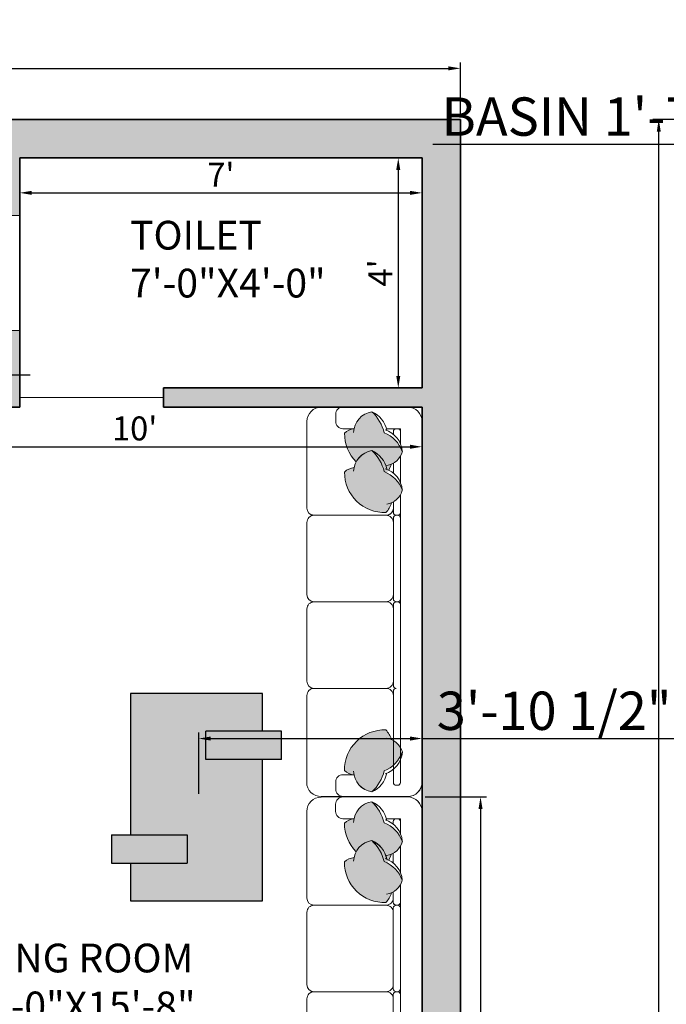
# Model space of a CAD drawing. Units: inches. Extents: x 3259 to 4981, y 1402 to 2026.
# Tile 4 of 11: x 3509 to 3644, y 1722 to 1928. Entities that reach past the tile are written whole.
import ezdxf

# ---------------------------------------------------------------- set-up
doc = ezdxf.new("R2010")
doc.units = ezdxf.units.IN
for name, color, linetype, lineweight in [('A-ANNO-DIMS', 2, 'Continuous', 13), ('A-AREA-IDEN', 7, 'Continuous', 18), ('A-DOOR', 3, 'Continuous', 18), ('A-FURN', 8, 'Continuous', 13), ('A-GLAZ', 4, 'Continuous', 18), ('A-WALL', 7, 'Continuous', 35), ('A-WALL-PATT', 252, 'Continuous', 13), ('parede', 7, 'Continuous', 30)]:
    doc.layers.add(name, color=color, linetype=linetype, lineweight=lineweight)
doc.styles.get("Standard").update_dxf_attribs({"font": 'arial.ttf'})
doc.dimstyles.new('ISO-25', dxfattribs={"dimtxt": 8, "dimasz": 2.5, "dimexe": 1.25, "dimexo": 0.625, "dimtad": 1, "dimdec": 1, "dimlunit": 3, "dimtxsty": 'Standard', "dimcen": 2.5, "dimclrd": 4, "dimclre": 4, "dimclrt": 1, "dimadec": 0, "dimazin": 0, "dimtfac": 1, "dimtdec": 1, "dimtmove": 0, "dimatfit": 3, "dimfxl": 1, "dimarcsym": 0})

# ---------------------------------------------------------------- blocks, each defined once
blk = doc.blocks.new('SOFA 1')
at = {"transparency": 33554687}
h = blk.add_hatch(color=256, dxfattribs=at)
h.dxf.hatch_style = 1
h.paths.add_polyline_path([(3769.65, 1307.6, 0.084911), (3767.15, 1309.12, 0.046133), (3766.46, 1311.13), (3759.18, 1311.13, 0.039409), (3758.92, 1310.24, 0.165523), (3756.31, 1309.02, 0.42585), (3767.59, 1297.95, 0.121928), (3769.15, 1300.58, 0.027403), (3769.65, 1300.83)])
h.paths.add_polyline_path([(3765.34, 1313.08), (3760.4, 1313.08, 0.097704), (3759.18, 1311.13), (3766.46, 1311.13, 0.04873)])
h.paths.add_polyline_path([(3763.76, 1314.88, 0.16488), (3760.4, 1313.08), (3765.34, 1313.08, 0.051917)])
h.paths.add_polyline_path([(3771.6, 1305.17, 0.090388), (3769.65, 1307.6), (3769.65, 1300.83, 0.136035), (3771.6, 1302.77)])
h = blk.add_hatch(color=256, dxfattribs=at)
h.dxf.hatch_style = 1
h.paths.add_polyline_path([(3723.52, 1308.63, 0.147724), (3717.76, 1305.24, 0.310469), (3722.42, 1300.4), (3722.42, 1300.25, 0.156703), (3723.62, 1297.8, 0.425821), (3734.69, 1309.08, 0.121928), (3732.05, 1310.63, 0.233216), (3728.6, 1313.59, 0.213835)])
h = blk.add_hatch(color=256, dxfattribs=at)
h.dxf.hatch_style = 1
h.paths.add_polyline_path([(3769.16, 1235.96, 0.122267), (3767.6, 1238.61, 0.425972), (3756.32, 1227.54, 0.165563), (3758.93, 1226.32, 0.309481), (3763.76, 1221.69, 0.002677), (3763.83, 1221.72, 0.146094), (3767.16, 1227.43, 0.212433), (3772.1, 1232.48, 0.235342)])
h = blk.add_hatch(color=256, dxfattribs=at)
h.dxf.hatch_style = 1
h.paths.add_polyline_path([(3769.16, 1225.36, 0.122267), (3767.6, 1228.01, 0.425972), (3756.32, 1216.94, 0.165563), (3758.93, 1215.72, 0.309481), (3763.76, 1211.09, 0.002677), (3763.83, 1211.12, 0.146094), (3767.16, 1216.83, 0.212433), (3772.1, 1221.88, 0.235342)])
for p, q in [((3720.45, 1316.13), (3773.58, 1316.13)), ((3777.51, 1312.19), (3777.51, 1213.72))]:
    blk.add_line(p, q, dxfattribs=at)
for points in [[(3763.76, 1314.88, -0.147724), (3767.15, 1309.12, -0.213355), (3772.1, 1304.05, 0.213355), (3767.15, 1309.12, 0.147724), (3763.76, 1314.88, -0.249545), (3767.86, 1309.77, 0.249545), (3763.77, 1314.89, 0.356779), (3758.8, 1309.23, -0.356779), (3763.76, 1314.88)], [(3717.76, 1305.24, -0.147724), (3723.52, 1308.63, -0.213355), (3728.59, 1313.59, 0.213355), (3723.52, 1308.63, 0.147724), (3717.76, 1305.24, -0.249545), (3722.86, 1309.34, 0.249545), (3717.75, 1305.25, 0.356779), (3723.4, 1300.28, -0.356779), (3717.76, 1305.24)], [(3728.58, 1313.6, -0.306333), (3732.42, 1309.31, 0.306333), (3728.58, 1313.6, 0.306674), (3722.72, 1308.89, -0.306674), (3728.58, 1313.6)], [(3734.69, 1309.08, -0.425972), (3723.62, 1297.8, -0.165552), (3722.4, 1300.4, 0.165552), (3723.62, 1297.79, 0.425972), (3734.69, 1309.07, 0.121514), (3732.07, 1310.63, -0.121514), (3734.69, 1309.08)], [(3767.6, 1297.95, -0.425972), (3756.31, 1309.01, -0.165552), (3758.92, 1310.24, 0.165552), (3756.31, 1309.02, 0.425972), (3767.59, 1297.95, 0.121514), (3769.14, 1300.57, -0.121514), (3767.6, 1297.95)], [(3772.11, 1304.06, -0.306333), (3767.83, 1300.22, 0.306333), (3772.11, 1304.06, 0.306674), (3767.4, 1309.91, -0.306674), (3772.11, 1304.06)], [(3770.44, 1286.63, -0.414214), (3769.66, 1287.4, 0.414214), (3770.44, 1286.63, 0.414214), (3769.66, 1285.83, -0.414214), (3770.44, 1286.63)], [(3748.01, 1262.99, -0.414214), (3746.05, 1264.95, 0.414214), (3748.01, 1262.97, 0.414213), (3746.05, 1261.01, -0.414213), (3748.01, 1262.99)], [(3770.44, 1262.99, -0.414214), (3769.66, 1263.77, 0.414214), (3770.44, 1262.99, 0.414214), (3769.66, 1262.19, -0.414214), (3770.44, 1262.99)], [(3770.83, 1262.97, -0.414214), (3771.61, 1262.19, 0.414214), (3770.83, 1262.99, 0.414214), (3771.61, 1263.77, -0.414214), (3770.83, 1262.97)], [(3748.01, 1239.35, -0.414214), (3746.05, 1241.31, 0.414214), (3748.01, 1239.33, 0.414213), (3746.05, 1237.37, -0.414213), (3748.01, 1239.35)], [(3767.7, 1239.33, -0.414214), (3769.66, 1237.37, 0.414214), (3767.7, 1239.35, 0.414214), (3769.66, 1241.31, -0.414214), (3767.7, 1239.33)], [(3770.44, 1239.35, -0.414214), (3769.66, 1240.13, 0.414214), (3770.44, 1239.33, 0.414214), (3769.66, 1238.55, -0.414214), (3770.44, 1239.35)], [(3770.83, 1239.33, -0.414214), (3771.61, 1238.55, 0.414214), (3770.83, 1239.35, 0.414214), (3771.61, 1240.13, -0.414214), (3770.83, 1239.33)], [(3756.32, 1227.54, -0.425972), (3767.6, 1238.61, -0.121514), (3769.16, 1235.98, 0.121514), (3767.6, 1238.61, 0.425972), (3756.32, 1227.54, 0.165552), (3758.93, 1226.32, -0.165552), (3756.32, 1227.54)], [(3772.1, 1232.5, -0.306674), (3767.41, 1226.64, 0.306674), (3772.1, 1232.5, 0.306333), (3767.84, 1236.34, -0.306333), (3772.1, 1232.5)], [(3763.78, 1221.67, 0.249545), (3767.87, 1226.78, -0.249545), (3763.76, 1221.69, -0.356779), (3758.81, 1227.32, 0.356779), (3763.77, 1221.68, 0.147724), (3767.16, 1227.43, 0.213355), (3772.11, 1232.51, -0.213355), (3767.16, 1227.43, -0.147724), (3763.78, 1221.67)], [(3756.32, 1216.94, -0.200233), (3759.49, 1224.76, 0.200233), (3756.32, 1216.94, 0.165552), (3758.93, 1215.72, -0.165552), (3756.32, 1216.94)], [(3772.1, 1221.9, -0.306674), (3767.41, 1216.04, 0.306674), (3772.1, 1221.9, -0.213355), (3767.16, 1216.83, -0.147724), (3763.77, 1211.08, 0.147724), (3767.15, 1216.83, 0.213355), (3772.1, 1221.9)], [(3763.76, 1211.09, -0.356779), (3758.81, 1216.72, 0.356779), (3763.76, 1211.09, 0.249545), (3767.87, 1216.18, -0.249545), (3763.76, 1211.09)]]:
    blk.add_lwpolyline(points, format="xyb", dxfattribs=at)
for points in [[(3716.51, 1312.2), (3716.51, 1291.44)], [(3722.42, 1313.08), (3722.42, 1309.23), (3722.42, 1313.08), (3726.57, 1313.08)], [(3729.85, 1313.08), (3745.25, 1313.08)], [(3746.01, 1312.3), (3746.01, 1288.55)], [(3768.11, 1313.08), (3746.78, 1313.08)], [(3771.6, 1313.08), (3767.75, 1313.08), (3771.6, 1313.08), (3771.6, 1308.93)], [(3769.66, 1287.39), (3769.65, 1312.3)], [(3771.6, 1313.08), (3771.61, 1233.74)], [(3723.21, 1311.13), (3723.93, 1311.13)], [(3731.82, 1311.13), (3745.25, 1311.13)], [(3746.01, 1310.97), (3746.01, 1311.36)], [(3768.87, 1311.13), (3746.78, 1311.13)], [(3769.65, 1309.43), (3769.65, 1308.71)], [(3746.01, 1288.54), (3746.01, 1308.23)], [(3722.42, 1300.39), (3722.42, 1297.33)], [(3720.45, 1295.38), (3718.48, 1295.38)], [(3720.45, 1287.5), (3744.09, 1287.5)], [(3747.99, 1286.6), (3767.69, 1286.6)], [(3769.66, 1263.75), (3769.66, 1285.81)], [(3746.02, 1284.63), (3746.02, 1264.94)], [(3769.66, 1277.18), (3769.66, 1263.75)], [(3746.02, 1260.99), (3746.02, 1241.3)], [(3747.99, 1262.97), (3767.69, 1262.97)], [(3769.66, 1240.12), (3769.66, 1262.18)], [(3770.43, 1262.97), (3770.82, 1262.97)], [(3746.02, 1237.36), (3746.02, 1213.74)], [(3747.99, 1239.33), (3767.69, 1239.33)], [(3769.66, 1235.71), (3769.66, 1238.54)], [(3770.43, 1239.33), (3770.82, 1239.33)], [(3771.61, 1223.14), (3771.61, 1230.47)], [(3769.66, 1225.11), (3769.66, 1227.82)], [(3767.76, 1215.72), (3771.61, 1215.72), (3771.61, 1219.84), (3771.61, 1215.72)], [(3755.86, 1215.72), (3758.92, 1215.72)], [(3769.66, 1216.5), (3769.66, 1217.22)], [(3753.91, 1211.77), (3753.91, 1213.74)], [(3749.97, 1209.8), (3773.58, 1209.8)]]:
    blk.add_lwpolyline(points, close=True, dxfattribs=at)
for points in [[(3770.43, 1313.08, 0.414214), (3769.65, 1312.3, -0.414214)], [(3771.6, 1312.3, 0.414214), (3770.82, 1313.08, -0.414214)], [(3722.42, 1311.91, 0.414214), (3723.2, 1311.13, -0.414214)], [(3716.51, 1297.34, 0.414214), (3718.47, 1295.38, -0.414214)], [(3720.44, 1295.38, 0.414214), (3722.4, 1297.34, -0.414214)], [(3716.51, 1291.45, 0.414212), (3720.44, 1287.52, -0.414212)], [(3746.03, 1288.56, 0.414214), (3747.99, 1286.6, 0.414213), (3746.03, 1284.64, -0.414213), (3747.99, 1286.6, -0.414214)], [(3769.66, 1284.64, 0.414214), (3767.7, 1286.6, 0.414214), (3769.66, 1288.56, -0.414214), (3767.7, 1286.6, -0.414214)], [(3769.66, 1261.01, 0.414214), (3767.7, 1262.97, 0.414214), (3769.66, 1264.93, -0.414214), (3767.7, 1262.97, -0.414214)], [(3769.16, 1225.36, 0.071861), (3768.39, 1227.01, -0.071861)], [(3772.13, 1221.9, 0.306333), (3767.84, 1225.74, -0.306333)], [(3755.87, 1215.72, 0.414214), (3753.91, 1213.76, -0.414214)], [(3769.66, 1216.52, 0.414214), (3770.44, 1215.74, -0.414214)], [(3770.83, 1215.74, 0.414214), (3771.61, 1216.52, -0.414214)], [(3746.05, 1213.76, 0.414212), (3749.98, 1209.82, -0.414212)], [(3755.87, 1209.8, -0.414214), (3753.91, 1211.76, 0.414214)]]:
    blk.add_lwpolyline(points, format="xyb", close=True, dxfattribs=at)
for centre, radius, start, end in [((3720.44, 1312.2), 3.93, 90.0002, 179.9998), ((3720.44, 1312.19), 3.94, 89.9158, 179.9154), ((3773.58, 1312.2), 3.93, 0.0002, 89.9998), ((3773.57, 1312.19), 3.94, 359.9158, 89.9154), ((3745.22, 1312.29), 0.789, 0.8425, 90.8425), ((3746.8, 1312.29), 0.789, 89.1575, 179.1575), ((3768.87, 1312.3), 0.777, 360, 90), ((3744.09, 1309.21), 1.92, 358.766, 90.5111), ((3745.24, 1311.91), 0.777, 270, 0), ((3745.24, 1311.91), 0.777, 270, 0), ((3746.79, 1311.91), 0.777, 180, 270), ((3746.79, 1311.91), 0.777, 180, 270), ((3747.93, 1309.21), 1.92, 89.4889, 181.234), ((3768.87, 1311.91), 0.777, 270, 0), ((3744.08, 1289.48), 1.96, 270, 360), ((3744.08, 1289.48), 1.96, 270, 360), ((3773.58, 1213.73), 3.93, 270.0002, 359.9998), ((3773.59, 1213.73), 3.93, 269.9156, 359.9152)]:
    blk.add_arc(centre, radius, start, end, dxfattribs=at)
blk = doc.blocks.new('Mesa de Centro Nalita')
at = {"layer": 'parede', "ltscale": 0.2}
h = blk.add_hatch(color=256, dxfattribs=at)
h.set_gradient(color1=(95, 72, 63), color2=(161, 128, 114), one_color=1, tint=0.54, name='INVCYLINDER')
h.paths.add_polyline_path([(0.35, -0.35), (0.05, -0.35), (0.05, -0.2), (0.35, -0.2), (0.35, 0), (-0.35, 0), (-0.35, -0.75), (-0.05, -0.75), (-0.05, -0.9), (-0.35, -0.9), (-0.35, -1.1), (0.35, -1.1)])
h = blk.add_hatch(color=256, dxfattribs=at)
h.set_gradient(color1=(95, 72, 63), color2=(161, 128, 114), one_color=1, tint=0.54, name='INVSPHERICAL')
h.paths.add_polyline_path([(0.05, -0.2), (0.05, -0.35), (0.45, -0.35), (0.45, -0.2)])
h = blk.add_hatch(color=256, dxfattribs=at)
h.set_gradient(color1=(95, 72, 63), color2=(161, 128, 114), one_color=1, tint=0.54, name='INVSPHERICAL')
h.paths.add_polyline_path([(-0.05, -0.9), (-0.05, -0.75), (-0.45, -0.75), (-0.45, -0.9)])
for p, q in [((0.35, 0), (-0.35, 0)), ((-0.35, 0), (-0.35, -0.75)), ((0.35, -0.2), (0.35, 0)), ((0.05, -0.35), (0.05, -0.2)), ((0.45, -0.2), (0.05, -0.2)), ((0.45, -0.35), (0.45, -0.2)), ((0.45, -0.35), (0.05, -0.35)), ((0.35, -1.1), (0.35, -0.35)), ((-0.45, -0.75), (-0.05, -0.75)), ((-0.45, -0.75), (-0.45, -0.9)), ((-0.05, -0.75), (-0.05, -0.9)), ((-0.45, -0.9), (-0.05, -0.9)), ((-0.35, -0.9), (-0.35, -1.1)), ((-0.35, -1.1), (0.35, -1.1))]:
    blk.add_line(p, q, dxfattribs=at)
blk = doc.blocks.new('*D21')
at = {"layer": 'A-ANNO-DIMS', "color": 0, "lineweight": -2, "transparency": 16777216}
for p, q in [((3301.16, 1907.74), (3301.16, 1919.06)), ((3303.66, 1917.81), (3598.66, 1917.81)), ((3601.16, 1907.74), (3601.16, 1919.06))]:
    blk.add_line(p, q, dxfattribs=at)
at = {"layer": 'A-ANNO-DIMS', "color": 0, "transparency": 16777216}
for points in [[(3303.66, 1918.23), (3303.66, 1917.39), (3301.16, 1917.81)], [(3598.66, 1918.23), (3598.66, 1917.39), (3601.16, 1917.81)]]:
    blk.add_solid(points, dxfattribs=at)
at = {"layer": 'Defpoints', "color": 0, "transparency": 16777216}
for p in [(3601.16, 1917.81), (3301.16, 1907.12), (3601.16, 1907.12)]:
    blk.add_point(p, dxfattribs=at)
at = {"layer": 'A-ANNO-DIMS', "color": 0, "transparency": 16777216, "insert": (3451.16, 1922.52), "char_height": 8, "attachment_point": 5}
blk.add_mtext("25'", dxfattribs=at)
blk = doc.blocks.new('*D25')
at = {"layer": 'A-ANNO-DIMS', "color": 0, "lineweight": -2, "transparency": 16777216}
for p, q in [((3593.16, 1846.49), (3593.16, 1837.58)), ((3473.16, 1843.37), (3473.16, 1837.58)), ((3475.66, 1838.83), (3590.66, 1838.83))]:
    blk.add_line(p, q, dxfattribs=at)
at = {"layer": 'A-ANNO-DIMS', "color": 0, "transparency": 16777216}
for points in [[(3475.66, 1839.25), (3475.66, 1838.42), (3473.16, 1838.83)], [(3590.66, 1839.25), (3590.66, 1838.42), (3593.16, 1838.83)]]:
    blk.add_solid(points, dxfattribs=at)
at = {"layer": 'Defpoints', "color": 0, "transparency": 16777216}
for p in [(3593.16, 1847.12), (3473.16, 1844), (3593.16, 1838.83)]:
    blk.add_point(p, dxfattribs=at)
at = {"layer": 'A-ANNO-DIMS', "color": 0, "transparency": 16777216, "insert": (3533.16, 1842.01), "char_height": 5, "attachment_point": 5}
blk.add_mtext("10'", dxfattribs=at)
blk = doc.blocks.new('*D39')
at = {"layer": 'A-ANNO-DIMS', "color": 0, "lineweight": -2, "transparency": 16777216}
for p, q in [((3509.16, 1898.49), (3509.16, 1890.58)), ((3593.16, 1898.49), (3593.16, 1890.58)), ((3511.66, 1891.83), (3590.66, 1891.83))]:
    blk.add_line(p, q, dxfattribs=at)
at = {"layer": 'A-ANNO-DIMS', "color": 0, "transparency": 16777216}
for points in [[(3511.66, 1892.25), (3511.66, 1891.41), (3509.16, 1891.83)], [(3590.66, 1892.25), (3590.66, 1891.41), (3593.16, 1891.83)]]:
    blk.add_solid(points, dxfattribs=at)
at = {"layer": 'Defpoints', "color": 0, "transparency": 16777216}
for p in [(3509.16, 1899.12), (3593.16, 1899.12), (3593.16, 1891.83)]:
    blk.add_point(p, dxfattribs=at)
at = {"layer": 'A-ANNO-DIMS', "color": 0, "transparency": 16777216, "insert": (3551.16, 1894.95), "char_height": 5, "attachment_point": 5}
blk.add_mtext("7'", dxfattribs=at)
blk = doc.blocks.new('*D40')
at = {"layer": 'A-ANNO-DIMS', "color": 0, "lineweight": -2, "transparency": 16777216}
for p, q in [((3592.54, 1899.12), (3586.94, 1899.12)), ((3588.19, 1896.62), (3588.19, 1853.62)), ((3592.54, 1851.12), (3586.94, 1851.12))]:
    blk.add_line(p, q, dxfattribs=at)
at = {"layer": 'A-ANNO-DIMS', "color": 0, "transparency": 16777216}
for points in [[(3587.77, 1896.62), (3588.61, 1896.62), (3588.19, 1899.12)], [(3587.77, 1853.62), (3588.61, 1853.62), (3588.19, 1851.12)]]:
    blk.add_solid(points, dxfattribs=at)
at = {"layer": 'Defpoints', "color": 0, "transparency": 16777216}
for p in [(3593.16, 1899.12), (3588.19, 1851.12), (3593.16, 1851.12)]:
    blk.add_point(p, dxfattribs=at)
at = {"layer": 'A-ANNO-DIMS', "color": 0, "transparency": 16777216, "insert": (3585.07, 1875.12), "char_height": 5, "attachment_point": 5, "rotation": 90}
blk.add_mtext("4'", dxfattribs=at)
blk = doc.blocks.new('SOFA-3SEAT')
at = {"transparency": 33554687}
h = blk.add_hatch(color=256, dxfattribs=at)
h.dxf.hatch_style = 1
h.paths.add_polyline_path([(17.7, 69.38, -0.122267), (16.5, 67.36, -0.425972), (7.88, 75.82, -0.165563), (9.87, 76.76, -0.309481), (13.57, 80.3, -0.002677), (13.62, 80.27, -0.146094), (16.16, 75.9, -0.212433), (19.95, 72.05, -0.235342)])
h = blk.add_hatch(color=256, dxfattribs=at)
h.dxf.hatch_style = 1
h.paths.add_polyline_path([(17.7, 61.28, -0.122267), (16.5, 59.26, -0.425972), (7.88, 67.72, -0.165563), (9.87, 68.65, -0.309481), (13.57, 72.19, -0.002677), (13.62, 72.17, -0.146094), (16.16, 67.8, -0.212433), (19.95, 63.95, -0.235342)])
h = blk.add_hatch(color=256, dxfattribs=at)
h.dxf.hatch_style = 1
h.paths.add_polyline_path([(18.07, 6.52, -0.084911), (16.16, 5.36, -0.046133), (15.63, 3.82), (10.07, 3.82, -0.039409), (9.87, 4.51, -0.165523), (7.87, 5.44, -0.42585), (16.5, 13.9, -0.121928), (17.69, 11.88, -0.027403), (18.07, 11.69)])
h.paths.add_polyline_path([(14.77, 2.33), (11, 2.33, -0.097704), (10.07, 3.82), (15.63, 3.82, -0.04873)])
h.paths.add_polyline_path([(13.57, 0.96, -0.16488), (11, 2.33), (14.77, 2.33, -0.051917)])
h.paths.add_polyline_path([(19.56, 8.38, -0.090388), (18.07, 6.52), (18.07, 11.69, -0.136035), (19.56, 10.21)])
blk.add_line((24.08, 3.01), (24.08, 78.28), dxfattribs=at)
blk.add_line((18.66, 2.33), (18.96, 2.33))
for points in [[(0.03, 78.26, -0.414212), (3.03, 81.26, 0.414212)], [(7.54, 81.28, 0.414214), (6.04, 79.78, -0.414214)], [(7.54, 76.76, -0.414214), (6.04, 78.26, 0.414214)], [(18.08, 76.15, -0.414214), (18.67, 76.74, 0.414214)], [(18.97, 76.74, -0.414214), (19.57, 76.15, 0.414214)], [(19.96, 72.03, -0.306333), (16.68, 69.1, 0.306333)], [(17.69, 69.39, -0.071861), (17.1, 68.12, 0.071861)], [(18.08, 42.14, -0.414214), (16.58, 40.64, -0.414214), (18.08, 39.14, 0.414214), (16.58, 40.64, 0.414214)], [(0.02, 21.07, -0.414214), (1.52, 22.57, -0.414213), (0.02, 24.07, 0.414213), (1.52, 22.57, 0.414214)], [(18.08, 24.07, -0.414214), (16.58, 22.57, -0.414214), (18.08, 21.07, 0.414214), (16.58, 22.57, 0.414214)], [(7.54, 4.54, 0.414214), (6.04, 3.04, -0.414214)], [(0, 2.93, 0.439287), (3.02, 0.02, -0.439287)], [(18.66, 2.33, -0.414214), (18.07, 2.93, 0.414214)], [(19.56, 2.93, -0.414214), (18.96, 2.33, 0.414214)], [(7.54, 0.02, -0.414214), (6.04, 1.52, 0.414214)]]:
    blk.add_lwpolyline(points, format="xyb", close=True, dxfattribs=at)
for points in [[(3.02, 81.28), (21.07, 81.28)], [(0.01, 60.21), (0.01, 78.27)], [(6.04, 79.77), (6.04, 78.27)], [(7.53, 76.76), (9.87, 76.76)], [(16.62, 76.76), (19.57, 76.76), (19.57, 73.6), (19.57, 76.76)], [(18.08, 76.16), (18.08, 75.61)], [(19.57, 71.08), (19.57, 65.48)], [(18.08, 69.58), (18.08, 67.5)], [(19.56, 2.93), (19.57, 62.98)], [(18.08, 61.47), (18.08, 59.31)], [(1.52, 58.71), (16.57, 58.71)], [(18.08, 58.1), (18.08, 41.24)], [(18.66, 58.71), (18.96, 58.71)], [(0.01, 42.15), (0.01, 57.2)], [(0.01, 24.08), (0.01, 39.13)], [(1.52, 40.64), (16.57, 40.64)], [(18.08, 29.77), (18.08, 40.04)], [(18.08, 40.04), (18.08, 23.17)], [(18.66, 40.64), (18.96, 40.64)], [(0, 2.93), (0, 21.08)], [(1.52, 22.57), (16.57, 22.57)], [(18.08, 21.97), (18.07, 2.93)], [(7.53, 4.54), (9.87, 4.54)], [(18.07, 5.12), (18.07, 5.67)], [(0, 3.95), (0, 3.64)], [(6.04, 1.52), (6.04, 3.03)], [(3.02, 0.02), (21.07, 0.02)]]:
    blk.add_lwpolyline(points, close=True, dxfattribs=at)
for points in [[(13.57, 80.3, 0.356779), (9.78, 75.99, -0.356779), (13.57, 80.3, -0.249545), (16.71, 76.4, 0.249545), (13.57, 80.3)], [(19.94, 72.03, 0.306674), (16.36, 76.51, -0.306674), (19.94, 72.03, 0.213355), (16.16, 75.9, 0.147724), (13.58, 80.3, -0.147724), (16.16, 75.91, -0.213355), (19.94, 72.03)], [(7.88, 75.82, 0.200233), (10.31, 69.84, -0.200233), (7.88, 75.82, -0.165552), (9.87, 76.76, 0.165552), (7.88, 75.82)], [(13.58, 72.21, -0.249545), (16.71, 68.3, 0.249545), (13.57, 72.19, 0.356779), (9.78, 67.89, -0.356779), (13.58, 72.2, -0.147724), (16.16, 67.8, -0.213355), (19.95, 63.92, 0.213355), (16.16, 67.8, 0.147724), (13.58, 72.21)], [(7.88, 67.72, 0.425972), (16.5, 59.26, 0.121514), (17.69, 61.27, -0.121514), (16.5, 59.26, -0.425972), (7.88, 67.72, -0.165552), (9.87, 68.65, 0.165552), (7.88, 67.72)], [(19.94, 63.93, 0.306674), (16.36, 68.41, -0.306674), (19.94, 63.93, -0.306333), (16.68, 61, 0.306333), (19.94, 63.93)], [(1.52, 58.69, 0.414214), (0.03, 57.19, -0.414214), (1.52, 58.71, -0.414213), (0.03, 60.21, 0.414213), (1.52, 58.69)], [(16.58, 58.71, 0.414214), (18.08, 60.21, -0.414214), (16.58, 58.69, -0.414214), (18.08, 57.19, 0.414214), (16.58, 58.71)], [(18.67, 58.69, 0.414214), (18.08, 58.1, -0.414214), (18.67, 58.71, -0.414214), (18.08, 59.3, 0.414214), (18.67, 58.69)], [(18.97, 58.71, 0.414214), (19.57, 59.3, -0.414214), (18.97, 58.69, -0.414214), (19.57, 58.1, 0.414214), (18.97, 58.71)], [(1.52, 40.62, 0.414214), (0.03, 39.12, -0.414214), (1.52, 40.64, -0.414213), (0.03, 42.14, 0.414213), (1.52, 40.62)], [(18.67, 40.62, 0.414214), (18.08, 40.03, -0.414214), (18.67, 40.62, -0.414214), (18.08, 41.23, 0.414214), (18.67, 40.62)], [(18.97, 40.64, 0.414214), (19.57, 41.23, -0.414214), (18.97, 40.62, -0.414214), (19.57, 40.03, 0.414214), (18.97, 40.64)], [(18.67, 22.55, 0.414214), (18.08, 21.96, -0.414214), (18.67, 22.55, -0.414214), (18.08, 23.17, 0.414214), (18.67, 22.55)], [(16.5, 13.9, 0.425972), (7.87, 5.44, 0.165552), (9.87, 4.51, -0.165552), (7.87, 5.44, -0.425972), (16.5, 13.9, -0.121514), (17.68, 11.89, 0.121514), (16.5, 13.9)], [(19.95, 9.23, 0.306333), (16.68, 12.16, -0.306333), (19.95, 9.23, -0.306674), (16.35, 4.75, 0.306674), (19.95, 9.23)], [(13.57, 0.96, 0.147724), (16.16, 5.36, 0.213355), (19.94, 9.23, -0.213355), (16.16, 5.36, -0.147724), (13.57, 0.96, 0.249545), (16.7, 4.86, -0.249545), (13.57, 0.95, -0.356779), (9.77, 5.27, 0.356779), (13.57, 0.96)]]:
    blk.add_lwpolyline(points, format="xyb", dxfattribs=at)
for centre, radius, start, end in [((21.08, 78.28), 3, 0.0848, 90.0844), ((21.07, 78.27), 3.01, 0.0002, 89.9998), ((21.07, 3.01), 3.01, 270.0002, 359.9998), ((21.07, 3.01), 3.01, 270.0846, 0.0842)]:
    blk.add_arc(centre, radius, start, end, dxfattribs=at)
blk = doc.blocks.new('VENT-24x4')
for p, q in [((0, 24), (4, 24)), ((2, 24), (2, 0)), ((0, 0), (4, 0))]:
    blk.add_line(p, q)
blk = doc.blocks.new('*D150')
at = {"layer": 'A-ANNO-DIMS', "color": 4, "lineweight": -2, "transparency": 16777216}
for p, q in [((3684.21, 1899.74), (3684.21, 1903.2)), ((3703.12, 1899.74), (3703.12, 1903.2)), ((3684.21, 1901.95), (3595.41, 1901.95)), ((3700.62, 1901.95), (3686.71, 1901.95))]:
    blk.add_line(p, q, dxfattribs=at)
at = {"layer": 'A-ANNO-DIMS', "color": 4, "transparency": 16777216}
for points in [[(3686.71, 1902.37), (3686.71, 1901.54), (3684.21, 1901.95)], [(3700.62, 1902.37), (3700.62, 1901.54), (3703.12, 1901.95)]]:
    blk.add_solid(points, dxfattribs=at)
at = {"layer": 'Defpoints', "color": 0, "transparency": 16777216}
for p in [(3684.21, 1901.95), (3684.21, 1899.12), (3703.12, 1899.12)]:
    blk.add_point(p, dxfattribs=at)
at = {"layer": 'A-ANNO-DIMS', "color": 1, "transparency": 16777216, "insert": (3638.56, 1906.71), "char_height": 8, "attachment_point": 5}
blk.add_mtext('BASIN 1\'-7" TYP.', dxfattribs=at)
blk = doc.blocks.new('*D156')
at = {"layer": 'A-ANNO-DIMS', "color": 4, "lineweight": -2, "transparency": 16777216}
for p, q in [((3593.79, 1765.74), (3606.61, 1765.74)), ((3605.36, 1763.24), (3605.36, 1686.95)), ((3593.79, 1684.45), (3606.61, 1684.45)), ((3605.36, 1684.45), (3605.36, 1579.8))]:
    blk.add_line(p, q, dxfattribs=at)
at = {"layer": 'A-ANNO-DIMS', "color": 4, "transparency": 16777216}
for points in [[(3604.94, 1763.24), (3605.78, 1763.24), (3605.36, 1765.74)], [(3604.94, 1686.95), (3605.78, 1686.95), (3605.36, 1684.45)]]:
    blk.add_solid(points, dxfattribs=at)
at = {"layer": 'Defpoints', "color": 0, "transparency": 16777216}
for p in [(3593.17, 1765.74), (3593.17, 1684.45), (3605.36, 1684.45)]:
    blk.add_point(p, dxfattribs=at)
at = {"layer": 'A-ANNO-DIMS', "color": 1, "transparency": 16777216, "insert": (3600.6, 1630.88), "char_height": 8, "attachment_point": 5, "rotation": 90}
blk.add_mtext('SOFA 6\'-9 1/2" TYP.', dxfattribs=at)
blk = doc.blocks.new('*D157')
at = {"layer": 'A-ANNO-DIMS', "color": 4, "lineweight": -2, "transparency": 16777216}
for p, q in [((3546.53, 1766.36), (3546.53, 1779.18)), ((3549.03, 1777.93), (3590.67, 1777.93)), ((3593.17, 1766.36), (3593.17, 1779.18)), ((3593.17, 1777.93), (3670.53, 1777.93))]:
    blk.add_line(p, q, dxfattribs=at)
at = {"layer": 'A-ANNO-DIMS', "color": 4, "transparency": 16777216}
for points in [[(3549.03, 1778.35), (3549.03, 1777.51), (3546.53, 1777.93)], [(3590.67, 1778.35), (3590.67, 1777.51), (3593.17, 1777.93)]]:
    blk.add_solid(points, dxfattribs=at)
at = {"layer": 'Defpoints', "color": 0, "transparency": 16777216}
for p in [(3593.17, 1777.93), (3546.53, 1765.74), (3593.17, 1765.74)]:
    blk.add_point(p, dxfattribs=at)
at = {"layer": 'A-ANNO-DIMS', "color": 1, "transparency": 16777216, "insert": (3633.1, 1782.69), "char_height": 8, "attachment_point": 5}
blk.add_mtext('3\'-10 1/2" TYP.', dxfattribs=at)
blk = doc.blocks.new('*D168')
at = {"layer": 'A-ANNO-DIMS', "color": 4, "lineweight": -2, "transparency": 16777216}
for p, q in [((3362.52, 1847.75), (3362.52, 1855.13)), ((3365.02, 1853.88), (3405.08, 1853.88)), ((3407.58, 1847.75), (3407.58, 1855.13)), ((3407.58, 1853.88), (3511.34, 1853.88))]:
    blk.add_line(p, q, dxfattribs=at)
at = {"layer": 'A-ANNO-DIMS', "color": 4, "transparency": 16777216}
for points in [[(3365.02, 1854.3), (3365.02, 1853.47), (3362.52, 1853.88)], [(3405.08, 1854.3), (3405.08, 1853.47), (3407.58, 1853.88)]]:
    blk.add_solid(points, dxfattribs=at)
at = {"layer": 'Defpoints', "color": 0, "transparency": 16777216}
for p in [(3407.58, 1853.88), (3362.52, 1847.13), (3407.58, 1847.13)]:
    blk.add_point(p, dxfattribs=at)
at = {"layer": 'A-ANNO-DIMS', "color": 1, "transparency": 16777216, "insert": (3460.71, 1858.6), "char_height": 8, "attachment_point": 5}
blk.add_mtext('WALL TV 3\'-9" TYP.', dxfattribs=at)
blk = doc.blocks.new('*D187')
at = {"layer": 'A-ANNO-DIMS', "color": 4, "lineweight": -2, "transparency": 16777216}
for p, q in [((3667.04, 1907.12), (3641.31, 1907.12)), ((3642.56, 1477.62), (3642.56, 1904.62)), ((3667.04, 1475.12), (3641.31, 1475.12))]:
    blk.add_line(p, q, dxfattribs=at)
at = {"layer": 'A-ANNO-DIMS', "color": 4, "transparency": 16777216}
for points in [[(3642.15, 1904.62), (3642.98, 1904.62), (3642.56, 1907.12)], [(3642.15, 1477.62), (3642.98, 1477.62), (3642.56, 1475.12)]]:
    blk.add_solid(points, dxfattribs=at)
at = {"layer": 'Defpoints', "color": 0, "transparency": 16777216}
for p in [(3642.56, 1907.12), (3667.66, 1907.12), (3667.66, 1475.12)]:
    blk.add_point(p, dxfattribs=at)
at = {"layer": 'A-ANNO-DIMS', "color": 1, "transparency": 16777216, "insert": (3637.85, 1691.12), "char_height": 8, "attachment_point": 5, "rotation": 90}
blk.add_mtext('36\'-0"', dxfattribs=at)

msp = doc.modelspace()

# ---------------------------------------------------------------- hatches: boundary and pattern name
at = {"layer": 'A-WALL-PATT'}
h = msp.add_hatch(color=256, dxfattribs=at)
h.dxf.hatch_style = 1
h.paths.add_polyline_path([(3601.16, 1907.12), (3301.16, 1907.12), (3301.16, 1475.12), (3398.16, 1475.12), (3398.16, 1483.12), (3309.16, 1483.12), (3309.16, 1579.12), (3421.16, 1579.12), (3421.16, 1583.12), (3309.16, 1583.12), (3309.16, 1721.12), (3433.16, 1721.12), (3433.16, 1725.12), (3309.16, 1725.12), (3309.16, 1899.12), (3345.16, 1899.12), (3345.16, 1881.12), (3349.16, 1881.12), (3349.16, 1899.12), (3429.16, 1899.12), (3429.16, 1887.12), (3433.16, 1887.12), (3433.16, 1899.12), (3505.16, 1899.12), (3505.16, 1887.12), (3509.16, 1887.12), (3509.16, 1899.12), (3593.16, 1899.12), (3593.16, 1851.12), (3539.16, 1851.12), (3539.16, 1847.12), (3593.16, 1847.12), (3593.16, 1659.12), (3587.16, 1659.12), (3587.16, 1651.12), (3593.16, 1651.12), (3593.16, 1475.12), (3601.16, 1475.12)])
h.paths.add_polyline_path([(3433.16, 1863.12), (3429.16, 1863.12), (3429.16, 1851.12), (3345.16, 1851.12), (3345.16, 1847.12), (3382.99, 1847.12), (3382.99, 1847.13), (3383.04, 1847.13), (3383.04, 1847.12), (3387.07, 1847.12), (3387.07, 1847.12), (3387.11, 1847.12), (3433.16, 1847.12)], flags=17)
h.paths.add_polyline_path([(3509.16, 1863.12), (3505.16, 1863.12), (3505.16, 1847.12), (3509.16, 1847.12)], flags=17)
h.paths.add_polyline_path([(3473.16, 1851.12), (3469.16, 1851.12), (3469.16, 1715.12), (3473.16, 1715.12), (3473.16, 1777.43), (3473.16, 1777.43), (3473.16, 1777.47), (3473.16, 1777.47), (3473.16, 1781.5), (3473.16, 1781.5), (3473.16, 1781.55)], flags=17)
h.paths.add_polyline_path([(3491.16, 1659.12), (3473.16, 1659.12), (3473.16, 1667.12), (3469.16, 1667.12), (3469.16, 1483.12), (3473.16, 1483.12), (3473.16, 1651.12), (3491.16, 1651.12)], flags=17)
h.paths.add_polyline_path([(3551.16, 1659.12), (3539.16, 1659.12), (3539.16, 1651.12), (3551.16, 1651.12)], flags=17)
h.paths.add_polyline_path([(3473.16, 1483.12), (3458.16, 1483.12), (3458.16, 1475.12), (3473.16, 1475.12)], flags=17)

# ---------------------------------------------------------------- linework, layer by layer
at = {"layer": 'A-DOOR'}
msp.add_line((3539.16, 1849.12), (3509.16, 1849.12), dxfattribs=at)
at = {"layer": 'A-WALL'}
for p, q in [((3509.16, 1899.12), (3509.16, 1847.12)), ((3509.16, 1899.12), (3593.16, 1899.12)), ((3593.16, 1899.12), (3593.16, 1851.12)), ((3539.16, 1851.12), (3539.16, 1847.12)), ((3539.16, 1851.12), (3593.16, 1851.12)), ((3505.16, 1847.12), (3509.16, 1847.12)), ((3539.16, 1847.12), (3593.16, 1847.12)), ((3593.16, 1847.12), (3593.16, 1659.12))]:
    msp.add_line(p, q, dxfattribs=at)
msp.add_lwpolyline([(3473.16, 1475.12), (3301.16, 1475.12), (3301.16, 1907.12), (3601.16, 1907.12), (3601.16, 1475.12), (3593.16, 1475.12)], dxfattribs=at)

# ---------------------------------------------------------------- block references
at = {"layer": 'A-FURN'}
msp.add_blockref('SOFA-3SEAT', (3569.09, 1765.84), dxfattribs=at)
at = {"layer": 'A-FURN', "xscale": 39.3701, "yscale": 39.3701, "zscale": 39.3701}
msp.add_blockref('Mesa de Centro Nalita', (3546.07, 1787.34), dxfattribs=at)
at = {"layer": 'A-FURN', "xscale": -0.7644053585719659, "yscale": 0.7644053585719659, "zscale": 0.7644053585719659, "rotation": 180}
msp.add_blockref('SOFA 1', (705.61, 2690.51), dxfattribs=at)
at = {"layer": 'A-GLAZ', "rotation": 180}
msp.add_blockref('VENT-24x4', (3509.16, 1887.12), dxfattribs=at)

# ---------------------------------------------------------------- texts
at = {"layer": 'A-AREA-IDEN', "char_height": 6, "attachment_point": 1}
for s, insert in [('TOILET\\P7\'-0"X4\'-0"', (3532.19, 1885.99)), ('LIVING ROOM\\P 10\'-0"X15\'-8"', (3494.1, 1735.12))]:
    msp.add_mtext_dynamic_manual_height_columns(s, width=127.3061, gutter_width=12.5, heights=[0], dxfattribs=dict(at, insert=insert))

# ---------------------------------------------------------------- dimensions: what is measured, and where the dimension line sits
at = {"layer": 'A-ANNO-DIMS'}
for base, p1, p2, override, picture, middle in [((3601.16, 1917.81), (3301.16, 1907.12), (3601.16, 1907.12), {"dimclrd": 0, "dimclre": 0, "dimclrt": 0}, '*D21', (3451.16, 1922.52)), ((3593.16, 1891.83), (3509.16, 1899.12), (3593.16, 1899.12), {"dimtxt": 5, "dimclrd": 0, "dimclre": 0, "dimclrt": 0}, '*D39', (3551.16, 1894.95)), ((3593.16, 1838.83), (3473.16, 1844), (3593.16, 1847.12), {"dimtxt": 5, "dimclrd": 0, "dimclre": 0, "dimclrt": 0}, '*D25', (3533.16, 1842.01))]:
    dim = msp.add_linear_dim(base=base, p1=p1, p2=p2, dimstyle='ISO-25', override=override, dxfattribs=at)
    dim.commit()
    dim.dimension.update_dxf_attribs({"geometry": picture, "text_midpoint": middle})
for base, p1, p2, angle, text, picture, middle in [((3684.21, 1901.95), (3703.12, 1899.12), (3684.21, 1899.12), 180, 'BASIN <> TYP.', '*D150', (3638.56, 1906.71)), ((3605.36, 1684.45), (3593.17, 1765.74), (3593.17, 1684.45), 270, 'SOFA <> TYP.', '*D156', (3600.6, 1630.88))]:
    dim = msp.add_linear_dim(base=base, p1=p1, p2=p2, angle=angle, text=text, dimstyle='ISO-25', override={"dimdec": 1, "dimlfac": 1, "dimrnd": 0, "dimzin": 1, "dimdsep": 46, "dimlunit": 4, "dimfrac": 2}, dxfattribs=at)
    dim.commit()
    dim.dimension.update_dxf_attribs({"geometry": picture, "text_midpoint": middle})
for base, p1, p2, override, picture, middle in [((3642.56, 1907.12), (3667.66, 1475.12), (3667.66, 1907.12), {"dimdec": 1, "dimlfac": 1, "dimrnd": 0, "dimzin": 1, "dimdsep": 46, "dimlunit": 4, "dimfrac": 2}, '*D187', (3637.85, 1691.12)), ((3588.19, 1851.12), (3593.16, 1899.12), (3593.16, 1851.12), {"dimtxt": 5, "dimclrd": 0, "dimclre": 0, "dimclrt": 0}, '*D40', (3585.07, 1875.12))]:
    dim = msp.add_linear_dim(base=base, p1=p1, p2=p2, angle=90, dimstyle='ISO-25', override=override, dxfattribs=at)
    dim.commit()
    dim.dimension.update_dxf_attribs({"geometry": picture, "text_midpoint": middle})
for base, p1, p2, text, picture, middle in [((3407.58, 1853.88), (3362.52, 1847.13), (3407.58, 1847.13), 'WALL TV <> TYP.', '*D168', (3460.71, 1858.6)), ((3593.17, 1777.93), (3546.53, 1765.74), (3593.17, 1765.74), '<> TYP.', '*D157', (3633.1, 1782.69))]:
    dim = msp.add_linear_dim(base=base, p1=p1, p2=p2, text=text, dimstyle='ISO-25', override={"dimdec": 1, "dimlfac": 1, "dimrnd": 0, "dimzin": 1, "dimdsep": 46, "dimlunit": 4, "dimfrac": 2}, dxfattribs=at)
    dim.commit()
    dim.dimension.update_dxf_attribs({"geometry": picture, "text_midpoint": middle})

doc.saveas('drawing.dxf')
